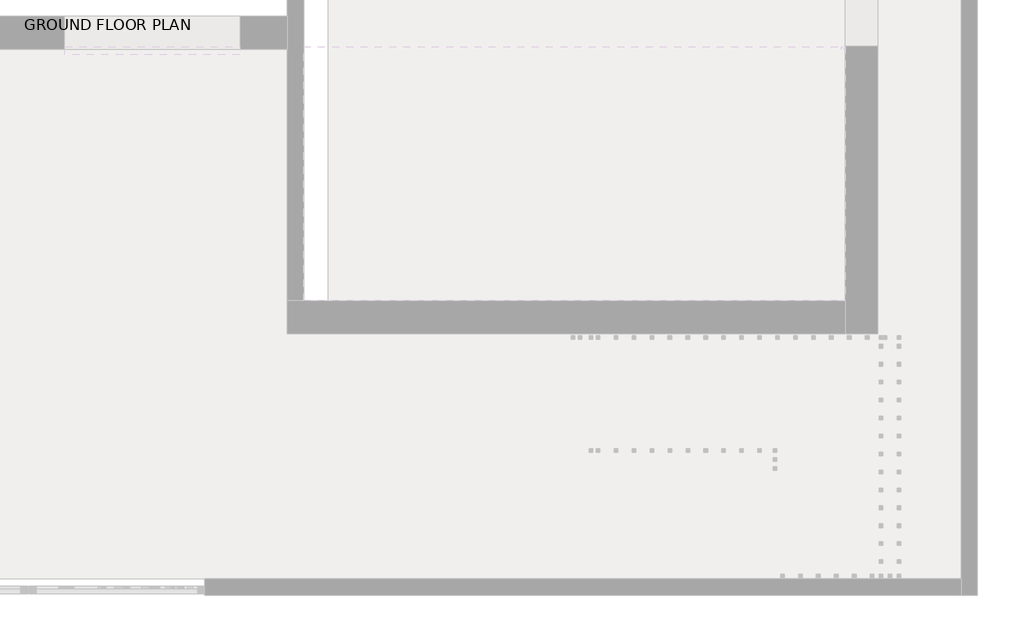
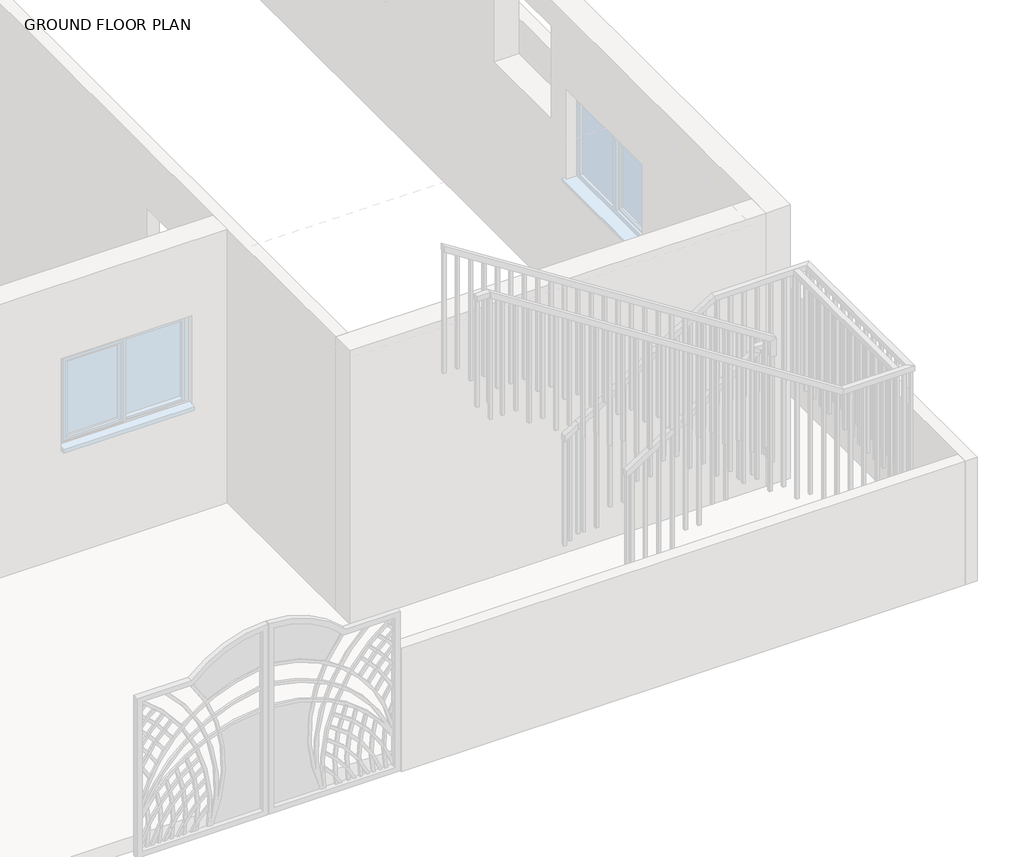
# One storey, part 14 of 23: 2 railings.
"""IFC4 building model written with IfcOpenShell, lengths in millimetres."""

from ifc_helpers import new_model, si_unit, frame, origin, place, context, project, spatial, polyline, outline, extrude, faceted_brep, element, save

model = new_model("IFC4")

# Units and contexts
model_context = context("Model", 3, world=origin())
ifc_project = project(units=[si_unit("LENGTHUNIT", "METRE", prefix="MILLI")], contexts=[model_context])

# Site, building, storey
site = spatial("IfcSite", under=ifc_project)
building = spatial("IfcBuilding", under=site)
storey = spatial("IfcBuildingStorey", under=building, Name="GROUND FLOOR PLAN", Elevation=487.68)

# Railings
placement = place(None, origin())
element("IfcRailing", 1, ObjectType="1100mm", at=placement, inside=storey, context=model_context, shape_type="SolidModel", body=[
    faceted_brep([(-8680.149573, -11007.9255223, 1912.8), (-8680.149573, -11007.9255223, 1853.4423995), (-8680.149573, -11057.9255223, 1853.4423995), (-8680.149573, -11057.9255223, 1912.8), (-7484.3306254, -11007.9255223, 2677.8717446), (-7434.3306254, -11007.9255223, 2650.5035914), (-7434.3306254, -11057.9255223, 2650.5035914), (-7484.3306254, -11057.9255223, 2677.8717446), (-7484.3306254, -11007.9255223, 2725.6), (-7434.3306254, -11007.9255223, 2675.6), (-7434.3306254, -11057.9255223, 2675.6), (-7484.3306254, -11057.9255223, 2725.6), (-7359.3306254, -11007.9255223, 2725.6), (-7359.3306254, -11007.9255223, 2675.6), (-7409.3306254, -11057.9255223, 2675.6), (-7409.3306254, -11057.9255223, 2725.6), (-7359.3306254, -11132.9255223, 2725.6), (-7359.3306254, -11132.9255223, 2675.6), (-7409.3306254, -11132.9255223, 2675.6), (-7409.3306254, -11132.9255223, 2725.6), (-7359.3306254, -11134.9255223, 2725.6), (-7409.3306254, -11134.9255223, 2725.6), (-7409.3306254, -11184.9255223, 2675.6), (-7359.3306254, -11184.9255223, 2675.6)], [[[0, 1, 2, 3]], [[1, 0, 4, 5]], [[2, 1, 5, 6]], [[3, 2, 6, 7]], [[0, 3, 7, 4]], [[5, 4, 8, 9]], [[6, 5, 9, 10]], [[7, 6, 10, 11]], [[4, 7, 11, 8]], [[9, 8, 12, 13]], [[10, 9, 13, 14]], [[11, 10, 14, 15]], [[8, 11, 15, 12]], [[13, 12, 16, 17]], [[14, 13, 17, 18]], [[15, 14, 18, 19]], [[12, 15, 19, 16]], [[20, 21, 22, 23]], [[17, 16, 20, 23]], [[18, 17, 23, 22]], [[19, 18, 22, 21]], [[16, 19, 21, 20]]]),
    faceted_brep([(-7359.3306254, -11134.9255223, 2725.6), (-7359.3306254, -11184.9255223, 2675.6), (-7409.3306254, -11184.9255223, 2675.6), (-7409.3306254, -11134.9255223, 2725.6), (-7359.3306254, -11134.9255223, 2855.9055527), (-7409.3306254, -11134.9255223, 2828.5415543), (-7409.3306254, -11184.9255223, 2828.5415543), (-7359.3306254, -11184.9255223, 2855.9055527)], [[[0, 1, 2, 3]], [[4, 5, 6, 7]], [[1, 0, 4, 7]], [[2, 1, 7, 6]], [[3, 2, 6, 5]], [[0, 3, 5, 4]]]),
    faceted_brep([(-7359.3306254, -11184.9255223, 2855.9055527), (-7409.3306254, -11184.9255223, 2828.5415543), (-7409.3306254, -11134.9255223, 2828.5415543), (-7359.3306254, -11134.9255223, 2855.9055527), (-10457.8773536, -11184.9255223, 4838.88), (-10457.8773536, -11134.9255223, 4838.88), (-10457.8773536, -11134.9255223, 4779.517542), (-10457.8773536, -11184.9255223, 4779.517542)], [[[0, 1, 2, 3]], [[4, 5, 6, 7]], [[1, 0, 4, 7]], [[2, 1, 7, 6]], [[3, 2, 6, 5]], [[0, 3, 5, 4]]]),
    extrude(outline(polyline([(3576.32, -10434.3306254), (4764.4483614, -10434.3306254), (4780.4475912, -10459.3306254), (3576.32, -10459.3306254), (3576.32, -10434.3306254)])), frame((0.0, -11172.4255223, 0.0), z_axis=(0.0, 1.0, 0.0), x_axis=(0.0, 0.0, 1.0)), (0.0, 0.0, 1.0), 25.0),
    extrude(outline(polyline([(3576.32, -10309.3306254), (4684.4522123, -10309.3306254), (4700.4514422, -10334.3306254), (3576.32, -10334.3306254), (3576.32, -10309.3306254)])), frame((0.0, -11172.4255223, 0.0), z_axis=(0.0, 1.0, 0.0), x_axis=(0.0, 0.0, 1.0)), (0.0, 0.0, 1.0), 25.0),
    extrude(outline(polyline([(3413.76, -10184.3306254), (4604.4560633, -10184.3306254), (4620.4552931, -10209.3306254), (3413.76, -10209.3306254), (3413.76, -10184.3306254)])), frame((0.0, -11172.4255223, 0.0), z_axis=(0.0, 1.0, 0.0), x_axis=(0.0, 0.0, 1.0)), (0.0, 0.0, 1.0), 25.0),
    extrude(outline(polyline([(3413.76, -10059.3306254), (4524.4599142, -10059.3306254), (4540.459144, -10084.3306254), (3413.76, -10084.3306254), (3413.76, -10059.3306254)])), frame((0.0, -11172.4255223, 0.0), z_axis=(0.0, 1.0, 0.0), x_axis=(0.0, 0.0, 1.0)), (0.0, 0.0, 1.0), 25.0),
    extrude(outline(polyline([(3251.2, -9934.3306254), (4444.4637652, -9934.3306254), (4460.462995, -9959.3306254), (3251.2, -9959.3306254), (3251.2, -9934.3306254)])), frame((0.0, -11172.4255223, 0.0), z_axis=(0.0, 1.0, 0.0), x_axis=(0.0, 0.0, 1.0)), (0.0, 0.0, 1.0), 25.0),
    extrude(outline(polyline([(3251.2, -9809.3306254), (4364.4676161, -9809.3306254), (4380.4668459, -9834.3306254), (3251.2, -9834.3306254), (3251.2, -9809.3306254)])), frame((0.0, -11172.4255223, 0.0), z_axis=(0.0, 1.0, 0.0), x_axis=(0.0, 0.0, 1.0)), (0.0, 0.0, 1.0), 25.0),
    extrude(outline(polyline([(3251.2, -9684.3306254), (4284.4714671, -9684.3306254), (4300.4706969, -9709.3306254), (3251.2, -9709.3306254), (3251.2, -9684.3306254)])), frame((0.0, -11172.4255223, 0.0), z_axis=(0.0, 1.0, 0.0), x_axis=(0.0, 0.0, 1.0)), (0.0, 0.0, 1.0), 25.0),
    extrude(outline(polyline([(3088.64, -9559.3306254), (4204.475318, -9559.3306254), (4220.4745478, -9584.3306254), (3088.64, -9584.3306254), (3088.64, -9559.3306254)])), frame((0.0, -11172.4255223, 0.0), z_axis=(0.0, 1.0, 0.0), x_axis=(0.0, 0.0, 1.0)), (0.0, 0.0, 1.0), 25.0),
    extrude(outline(polyline([(3088.64, -9434.3306254), (4124.479169, -9434.3306254), (4140.4783988, -9459.3306254), (3088.64, -9459.3306254), (3088.64, -9434.3306254)])), frame((0.0, -11172.4255223, 0.0), z_axis=(0.0, 1.0, 0.0), x_axis=(0.0, 0.0, 1.0)), (0.0, 0.0, 1.0), 25.0),
    extrude(outline(polyline([(2926.08, -9309.3306254), (4044.4830199, -9309.3306254), (4060.4822497, -9334.3306254), (2926.08, -9334.3306254), (2926.08, -9309.3306254)])), frame((0.0, -11172.4255223, 0.0), z_axis=(0.0, 1.0, 0.0), x_axis=(0.0, 0.0, 1.0)), (0.0, 0.0, 1.0), 25.0),
    extrude(outline(polyline([(2926.08, -9184.3306254), (3964.4868709, -9184.3306254), (3980.4861007, -9209.3306254), (2926.08, -9209.3306254), (2926.08, -9184.3306254)])), frame((0.0, -11172.4255223, 0.0), z_axis=(0.0, 1.0, 0.0), x_axis=(0.0, 0.0, 1.0)), (0.0, 0.0, 1.0), 25.0),
    extrude(outline(polyline([(2763.52, -9059.3306254), (3884.4907218, -9059.3306254), (3900.4899516, -9084.3306254), (2763.52, -9084.3306254), (2763.52, -9059.3306254)])), frame((0.0, -11172.4255223, 0.0), z_axis=(0.0, 1.0, 0.0), x_axis=(0.0, 0.0, 1.0)), (0.0, 0.0, 1.0), 25.0),
    extrude(outline(polyline([(2763.52, -8934.3306254), (3804.4945728, -8934.3306254), (3820.4938026, -8959.3306254), (2763.52, -8959.3306254), (2763.52, -8934.3306254)])), frame((0.0, -11172.4255223, 0.0), z_axis=(0.0, 1.0, 0.0), x_axis=(0.0, 0.0, 1.0)), (0.0, 0.0, 1.0), 25.0),
    extrude(outline(polyline([(2600.96, -8809.3306254), (3724.4984237, -8809.3306254), (3740.4976535, -8834.3306254), (2600.96, -8834.3306254), (2600.96, -8809.3306254)])), frame((0.0, -11172.4255223, 0.0), z_axis=(0.0, 1.0, 0.0), x_axis=(0.0, 0.0, 1.0)), (0.0, 0.0, 1.0), 25.0),
    extrude(outline(polyline([(2600.96, -8684.3306254), (3644.5022747, -8684.3306254), (3660.5015045, -8709.3306254), (2600.96, -8709.3306254), (2600.96, -8684.3306254)])), frame((0.0, -11172.4255223, 0.0), z_axis=(0.0, 1.0, 0.0), x_axis=(0.0, 0.0, 1.0)), (0.0, 0.0, 1.0), 25.0),
    extrude(outline(polyline([(2438.4, -8559.3306254), (3564.5061256, -8559.3306254), (3580.5053554, -8584.3306254), (2438.4, -8584.3306254), (2438.4, -8559.3306254)])), frame((0.0, -11172.4255223, 0.0), z_axis=(0.0, 1.0, 0.0), x_axis=(0.0, 0.0, 1.0)), (0.0, 0.0, 1.0), 25.0),
    extrude(outline(polyline([(2438.4, -8434.3306254), (3484.5099766, -8434.3306254), (3500.5092064, -8459.3306254), (2438.4, -8459.3306254), (2438.4, -8434.3306254)])), frame((0.0, -11172.4255223, 0.0), z_axis=(0.0, 1.0, 0.0), x_axis=(0.0, 0.0, 1.0)), (0.0, 0.0, 1.0), 25.0),
    extrude(outline(polyline([(2275.84, -8309.3306254), (3404.5138275, -8309.3306254), (3420.5130573, -8334.3306254), (2275.84, -8334.3306254), (2275.84, -8309.3306254)])), frame((0.0, -11172.4255223, 0.0), z_axis=(0.0, 1.0, 0.0), x_axis=(0.0, 0.0, 1.0)), (0.0, 0.0, 1.0), 25.0),
    extrude(outline(polyline([(2275.84, -8184.3306254), (3324.5176785, -8184.3306254), (3340.5169083, -8209.3306254), (2275.84, -8209.3306254), (2275.84, -8184.3306254)])), frame((0.0, -11172.4255223, 0.0), z_axis=(0.0, 1.0, 0.0), x_axis=(0.0, 0.0, 1.0)), (0.0, 0.0, 1.0), 25.0),
    extrude(outline(polyline([(2113.28, -8059.3306254), (3244.5215294, -8059.3306254), (3260.5207592, -8084.3306254), (2113.28, -8084.3306254), (2113.28, -8059.3306254)])), frame((0.0, -11172.4255223, 0.0), z_axis=(0.0, 1.0, 0.0), x_axis=(0.0, 0.0, 1.0)), (0.0, 0.0, 1.0), 25.0),
    extrude(outline(polyline([(2113.28, -7934.3306254), (3164.5253804, -7934.3306254), (3180.5246102, -7959.3306254), (2113.28, -7959.3306254), (2113.28, -7934.3306254)])), frame((0.0, -11172.4255223, 0.0), z_axis=(0.0, 1.0, 0.0), x_axis=(0.0, 0.0, 1.0)), (0.0, 0.0, 1.0), 25.0),
    extrude(outline(polyline([(1950.72, -7809.3306254), (3084.5292313, -7809.3306254), (3100.5284611, -7834.3306254), (1950.72, -7834.3306254), (1950.72, -7809.3306254)])), frame((0.0, -11172.4255223, 0.0), z_axis=(0.0, 1.0, 0.0), x_axis=(0.0, 0.0, 1.0)), (0.0, 0.0, 1.0), 25.0),
    extrude(outline(polyline([(1950.72, -7684.3306254), (3004.5330823, -7684.3306254), (3020.5323121, -7709.3306254), (1950.72, -7709.3306254), (1950.72, -7684.3306254)])), frame((0.0, -11172.4255223, 0.0), z_axis=(0.0, 1.0, 0.0), x_axis=(0.0, 0.0, 1.0)), (0.0, 0.0, 1.0), 25.0),
    extrude(outline(polyline([(1788.16, -7559.3306254), (2924.5369332, -7559.3306254), (2940.536163, -7584.3306254), (1788.16, -7584.3306254), (1788.16, -7559.3306254)])), frame((0.0, -11172.4255223, 0.0), z_axis=(0.0, 1.0, 0.0), x_axis=(0.0, 0.0, 1.0)), (0.0, 0.0, 1.0), 25.0),
    extrude(outline(polyline([(1788.16, -7434.3306254), (2844.5407841, -7434.3306254), (2860.540014, -7459.3306254), (1788.16, -7459.3306254), (1788.16, -7434.3306254)])), frame((0.0, -11172.4255223, 0.0), z_axis=(0.0, 1.0, 0.0), x_axis=(0.0, 0.0, 1.0)), (0.0, 0.0, 1.0), 25.0),
    extrude(outline(polyline([(-7396.8306254, -11082.9255223), (-7371.8306254, -11082.9255223), (-7371.8306254, -11107.9255223), (-7396.8306254, -11107.9255223), (-7396.8306254, -11082.9255223)])), frame((0.0, 0.0, 1625.6), z_axis=(0.0, 0.0, 1.0), x_axis=(1.0, 0.0, 0.0)), (0.0, 0.0, 1.0), 1050.0),
    extrude(outline(polyline([(2605.1944115, -7505.149573), (1463.04, -7505.149573), (1463.04, -7480.149573), (2621.1891352, -7480.149573), (2605.1944115, -7505.149573)])), frame((0.0, -11045.4255223, 0.0), z_axis=(0.0, 1.0, 0.0), x_axis=(0.0, 0.0, 1.0)), (0.0, 0.0, 1.0), 25.0),
    extrude(outline(polyline([(2525.2207932, -7630.149573), (1463.04, -7630.149573), (1463.04, -7605.149573), (2541.2155169, -7605.149573), (2525.2207932, -7630.149573)])), frame((0.0, -11045.4255223, 0.0), z_axis=(0.0, 1.0, 0.0), x_axis=(0.0, 0.0, 1.0)), (0.0, 0.0, 1.0), 25.0),
    extrude(outline(polyline([(2445.2471749, -7755.149573), (1300.48, -7755.149573), (1300.48, -7730.149573), (2461.2418986, -7730.149573), (2445.2471749, -7755.149573)])), frame((0.0, -11045.4255223, 0.0), z_axis=(0.0, 1.0, 0.0), x_axis=(0.0, 0.0, 1.0)), (0.0, 0.0, 1.0), 25.0),
    extrude(outline(polyline([(2365.2735566, -7880.149573), (1300.48, -7880.149573), (1300.48, -7855.149573), (2381.2682803, -7855.149573), (2365.2735566, -7880.149573)])), frame((0.0, -11045.4255223, 0.0), z_axis=(0.0, 1.0, 0.0), x_axis=(0.0, 0.0, 1.0)), (0.0, 0.0, 1.0), 25.0),
    extrude(outline(polyline([(2285.2999383, -8005.149573), (1137.92, -8005.149573), (1137.92, -7980.149573), (2301.294662, -7980.149573), (2285.2999383, -8005.149573)])), frame((0.0, -11045.4255223, 0.0), z_axis=(0.0, 1.0, 0.0), x_axis=(0.0, 0.0, 1.0)), (0.0, 0.0, 1.0), 25.0),
    extrude(outline(polyline([(2205.32632, -8130.149573), (1137.92, -8130.149573), (1137.92, -8105.149573), (2221.3210437, -8105.149573), (2205.32632, -8130.149573)])), frame((0.0, -11045.4255223, 0.0), z_axis=(0.0, 1.0, 0.0), x_axis=(0.0, 0.0, 1.0)), (0.0, 0.0, 1.0), 25.0),
    extrude(outline(polyline([(2125.3527017, -8255.149573), (975.36, -8255.149573), (975.36, -8230.149573), (2141.3474254, -8230.149573), (2125.3527017, -8255.149573)])), frame((0.0, -11045.4255223, 0.0), z_axis=(0.0, 1.0, 0.0), x_axis=(0.0, 0.0, 1.0)), (0.0, 0.0, 1.0), 25.0),
    extrude(outline(polyline([(2045.3790834, -8380.149573), (975.36, -8380.149573), (975.36, -8355.149573), (2061.3738071, -8355.149573), (2045.3790834, -8380.149573)])), frame((0.0, -11045.4255223, 0.0), z_axis=(0.0, 1.0, 0.0), x_axis=(0.0, 0.0, 1.0)), (0.0, 0.0, 1.0), 25.0),
    extrude(outline(polyline([(1965.4054651, -8505.149573), (812.8, -8505.149573), (812.8, -8480.149573), (1981.4001888, -8480.149573), (1965.4054651, -8505.149573)])), frame((0.0, -11045.4255223, 0.0), z_axis=(0.0, 1.0, 0.0), x_axis=(0.0, 0.0, 1.0)), (0.0, 0.0, 1.0), 25.0),
    extrude(outline(polyline([(1885.4318468, -8630.149573), (812.8, -8630.149573), (812.8, -8605.149573), (1901.4265705, -8605.149573), (1885.4318468, -8630.149573)])), frame((0.0, -11045.4255223, 0.0), z_axis=(0.0, 1.0, 0.0), x_axis=(0.0, 0.0, 1.0)), (0.0, 0.0, 1.0), 25.0),
    extrude(outline(polyline([(-7396.8306254, -11147.4255223), (-7371.8306254, -11147.4255223), (-7371.8306254, -11172.4255223), (-7396.8306254, -11172.4255223), (-7396.8306254, -11147.4255223)])), frame((0.0, 0.0, 1625.6), z_axis=(0.0, 0.0, 1.0), x_axis=(1.0, 0.0, 0.0)), (0.0, 0.0, 1.0), 1050.0),
    extrude(outline(polyline([(-7396.8306254, -11045.4255223), (-7396.8306254, -11020.4255223), (-7371.8306254, -11020.4255223), (-7371.8306254, -11045.4255223), (-7396.8306254, -11045.4255223)])), frame((0.0, 0.0, 1625.6), z_axis=(0.0, 0.0, 1.0), x_axis=(1.0, 0.0, 0.0)), (0.0, 0.0, 1.0), 1050.0),
    extrude(outline(polyline([(3576.32, -10432.8773536), (4763.5183122, -10432.8773536), (4779.517542, -10457.8773536), (3576.32, -10457.8773536), (3576.32, -10432.8773536)])), frame((0.0, -11172.4255223, 0.0), z_axis=(0.0, 1.0, 0.0), x_axis=(0.0, 0.0, 1.0)), (0.0, 0.0, 1.0), 25.0),
    extrude(outline(polyline([(1853.4423995, -8680.149573), (812.8, -8680.149573), (812.8, -8655.149573), (1869.4371231, -8655.149573), (1853.4423995, -8680.149573)])), frame((0.0, -11045.4255223, 0.0), z_axis=(0.0, 1.0, 0.0), x_axis=(0.0, 0.0, 1.0)), (0.0, 0.0, 1.0), 25.0),
])
element("IfcRailing", 2, ObjectType="1100mm", at=placement, inside=storey, context=model_context, shape_type="SolidModel", body=[
    faceted_brep([(-8680.149573, -10220.0521308, 1912.8), (-8680.149573, -10220.0521308, 1853.4423995), (-8680.149573, -10270.0521308, 1853.4423995), (-8680.149573, -10270.0521308, 1912.8), (-7409.7306254, -10220.0521308, 2725.6), (-7395.1045513, -10220.0521308, 2675.6), (-7395.1045513, -10270.0521308, 2675.6), (-7409.7306254, -10270.0521308, 2725.6), (-6495.8132565, -10220.0521308, 2725.6), (-6495.8132565, -10220.0521308, 2675.6), (-6545.8132565, -10270.0521308, 2675.6), (-6545.8132565, -10270.0521308, 2725.6), (-6495.8132565, -11933.6860066, 2725.6), (-6495.8132565, -11933.6860066, 2675.6), (-6545.8132565, -11883.6860066, 2675.6), (-6545.8132565, -11883.6860066, 2725.6), (-7155.718398, -11933.6860066, 2725.6), (-7170.3479429, -11933.6860066, 2675.6), (-7170.3479429, -11883.6860066, 2675.6), (-7155.718398, -11883.6860066, 2725.6), (-10457.8773536, -11933.6860066, 4838.88), (-10457.8773536, -11883.6860066, 4838.88), (-10457.8773536, -11883.6860066, 4779.517542), (-10457.8773536, -11933.6860066, 4779.517542)], [[[0, 1, 2, 3]], [[1, 0, 4, 5]], [[2, 1, 5, 6]], [[3, 2, 6, 7]], [[0, 3, 7, 4]], [[5, 4, 8, 9]], [[6, 5, 9, 10]], [[7, 6, 10, 11]], [[4, 7, 11, 8]], [[9, 8, 12, 13]], [[10, 9, 13, 14]], [[11, 10, 14, 15]], [[8, 11, 15, 12]], [[13, 12, 16, 17]], [[14, 13, 17, 18]], [[15, 14, 18, 19]], [[12, 15, 19, 16]], [[20, 21, 22, 23]], [[17, 16, 20, 23]], [[18, 17, 23, 22]], [[19, 18, 22, 21]], [[16, 19, 21, 20]]]),
    extrude(outline(polyline([(4691.8007425, -10320.8132565), (4707.7999723, -10345.8132565), (3576.32, -10345.8132565), (3576.32, -10320.8132565), (4691.8007425, -10320.8132565)])), frame((0.0, -11921.1860066, 0.0), z_axis=(0.0, 1.0, 0.0), x_axis=(0.0, 0.0, 1.0)), (0.0, 0.0, 1.0), 25.0),
    extrude(outline(polyline([(4611.8045935, -10195.8132565), (4627.8038233, -10220.8132565), (3576.32, -10220.8132565), (3576.32, -10195.8132565), (4611.8045935, -10195.8132565)])), frame((0.0, -11921.1860066, 0.0), z_axis=(0.0, 1.0, 0.0), x_axis=(0.0, 0.0, 1.0)), (0.0, 0.0, 1.0), 25.0),
    extrude(outline(polyline([(4531.8084444, -10070.8132565), (4547.8076742, -10095.8132565), (3413.76, -10095.8132565), (3413.76, -10070.8132565), (4531.8084444, -10070.8132565)])), frame((0.0, -11921.1860066, 0.0), z_axis=(0.0, 1.0, 0.0), x_axis=(0.0, 0.0, 1.0)), (0.0, 0.0, 1.0), 25.0),
    extrude(outline(polyline([(4451.8122954, -9945.8132565), (4467.8115252, -9970.8132565), (3413.76, -9970.8132565), (3413.76, -9945.8132565), (4451.8122954, -9945.8132565)])), frame((0.0, -11921.1860066, 0.0), z_axis=(0.0, 1.0, 0.0), x_axis=(0.0, 0.0, 1.0)), (0.0, 0.0, 1.0), 25.0),
    extrude(outline(polyline([(4371.8161463, -9820.8132565), (4387.8153761, -9845.8132565), (3251.2, -9845.8132565), (3251.2, -9820.8132565), (4371.8161463, -9820.8132565)])), frame((0.0, -11921.1860066, 0.0), z_axis=(0.0, 1.0, 0.0), x_axis=(0.0, 0.0, 1.0)), (0.0, 0.0, 1.0), 25.0),
    extrude(outline(polyline([(4291.8423995, -9695.8132565), (4307.8371231, -9720.8132565), (3251.2, -9720.8132565), (3251.2, -9695.8132565), (4291.8423995, -9695.8132565)])), frame((0.0, -11921.1860066, 0.0), z_axis=(0.0, 1.0, 0.0), x_axis=(0.0, 0.0, 1.0)), (0.0, 0.0, 1.0), 25.0),
    extrude(outline(polyline([(4211.8238482, -9570.8132565), (4227.823078, -9595.8132565), (3088.64, -9595.8132565), (3088.64, -9570.8132565), (4211.8238482, -9570.8132565)])), frame((0.0, -11921.1860066, 0.0), z_axis=(0.0, 1.0, 0.0), x_axis=(0.0, 0.0, 1.0)), (0.0, 0.0, 1.0), 25.0),
    extrude(outline(polyline([(4131.8276992, -9445.8132565), (4147.826929, -9470.8132565), (3088.64, -9470.8132565), (3088.64, -9445.8132565), (4131.8276992, -9445.8132565)])), frame((0.0, -11921.1860066, 0.0), z_axis=(0.0, 1.0, 0.0), x_axis=(0.0, 0.0, 1.0)), (0.0, 0.0, 1.0), 25.0),
    extrude(outline(polyline([(4051.8315501, -9320.8132565), (4067.8307799, -9345.8132565), (2926.08, -9345.8132565), (2926.08, -9320.8132565), (4051.8315501, -9320.8132565)])), frame((0.0, -11921.1860066, 0.0), z_axis=(0.0, 1.0, 0.0), x_axis=(0.0, 0.0, 1.0)), (0.0, 0.0, 1.0), 25.0),
    extrude(outline(polyline([(3971.835401, -9195.8132565), (3987.8346309, -9220.8132565), (2926.08, -9220.8132565), (2926.08, -9195.8132565), (3971.835401, -9195.8132565)])), frame((0.0, -11921.1860066, 0.0), z_axis=(0.0, 1.0, 0.0), x_axis=(0.0, 0.0, 1.0)), (0.0, 0.0, 1.0), 25.0),
    extrude(outline(polyline([(3891.839252, -9070.8132565), (3907.8384818, -9095.8132565), (2763.52, -9095.8132565), (2763.52, -9070.8132565), (3891.839252, -9070.8132565)])), frame((0.0, -11921.1860066, 0.0), z_axis=(0.0, 1.0, 0.0), x_axis=(0.0, 0.0, 1.0)), (0.0, 0.0, 1.0), 25.0),
    extrude(outline(polyline([(3811.8431029, -8945.8132565), (3827.8423328, -8970.8132565), (2763.52, -8970.8132565), (2763.52, -8945.8132565), (3811.8431029, -8945.8132565)])), frame((0.0, -11921.1860066, 0.0), z_axis=(0.0, 1.0, 0.0), x_axis=(0.0, 0.0, 1.0)), (0.0, 0.0, 1.0), 25.0),
    extrude(outline(polyline([(3731.8469539, -8820.8132565), (3747.8461837, -8845.8132565), (2600.96, -8845.8132565), (2600.96, -8820.8132565), (3731.8469539, -8820.8132565)])), frame((0.0, -11921.1860066, 0.0), z_axis=(0.0, 1.0, 0.0), x_axis=(0.0, 0.0, 1.0)), (0.0, 0.0, 1.0), 25.0),
    extrude(outline(polyline([(3651.8508048, -8695.8132565), (3667.8500347, -8720.8132565), (2600.96, -8720.8132565), (2600.96, -8695.8132565), (3651.8508048, -8695.8132565)])), frame((0.0, -11921.1860066, 0.0), z_axis=(0.0, 1.0, 0.0), x_axis=(0.0, 0.0, 1.0)), (0.0, 0.0, 1.0), 25.0),
    extrude(outline(polyline([(3571.8546558, -8570.8132565), (3587.8538856, -8595.8132565), (2438.4, -8595.8132565), (2438.4, -8570.8132565), (3571.8546558, -8570.8132565)])), frame((0.0, -11921.1860066, 0.0), z_axis=(0.0, 1.0, 0.0), x_axis=(0.0, 0.0, 1.0)), (0.0, 0.0, 1.0), 25.0),
    extrude(outline(polyline([(3491.8585067, -8445.8132565), (3507.8577365, -8470.8132565), (2438.4, -8470.8132565), (2438.4, -8445.8132565), (3491.8585067, -8445.8132565)])), frame((0.0, -11921.1860066, 0.0), z_axis=(0.0, 1.0, 0.0), x_axis=(0.0, 0.0, 1.0)), (0.0, 0.0, 1.0), 25.0),
    extrude(outline(polyline([(3411.8623577, -8320.8132565), (3427.8615875, -8345.8132565), (2275.84, -8345.8132565), (2275.84, -8320.8132565), (3411.8623577, -8320.8132565)])), frame((0.0, -11921.1860066, 0.0), z_axis=(0.0, 1.0, 0.0), x_axis=(0.0, 0.0, 1.0)), (0.0, 0.0, 1.0), 25.0),
    extrude(outline(polyline([(3331.8662086, -8195.8132565), (3347.8654384, -8220.8132565), (2275.84, -8220.8132565), (2275.84, -8195.8132565), (3331.8662086, -8195.8132565)])), frame((0.0, -11921.1860066, 0.0), z_axis=(0.0, 1.0, 0.0), x_axis=(0.0, 0.0, 1.0)), (0.0, 0.0, 1.0), 25.0),
    extrude(outline(polyline([(3251.8700596, -8070.8132565), (3267.8692894, -8095.8132565), (2113.28, -8095.8132565), (2113.28, -8070.8132565), (3251.8700596, -8070.8132565)])), frame((0.0, -11921.1860066, 0.0), z_axis=(0.0, 1.0, 0.0), x_axis=(0.0, 0.0, 1.0)), (0.0, 0.0, 1.0), 25.0),
    extrude(outline(polyline([(3171.8739105, -7945.8132565), (3187.8731403, -7970.8132565), (2113.28, -7970.8132565), (2113.28, -7945.8132565), (3171.8739105, -7945.8132565)])), frame((0.0, -11921.1860066, 0.0), z_axis=(0.0, 1.0, 0.0), x_axis=(0.0, 0.0, 1.0)), (0.0, 0.0, 1.0), 25.0),
    extrude(outline(polyline([(3091.8777615, -7820.8132565), (3107.8769913, -7845.8132565), (1950.72, -7845.8132565), (1950.72, -7820.8132565), (3091.8777615, -7820.8132565)])), frame((0.0, -11921.1860066, 0.0), z_axis=(0.0, 1.0, 0.0), x_axis=(0.0, 0.0, 1.0)), (0.0, 0.0, 1.0), 25.0),
    extrude(outline(polyline([(3011.8816124, -7695.8132565), (3027.8808422, -7720.8132565), (1950.72, -7720.8132565), (1950.72, -7695.8132565), (3011.8816124, -7695.8132565)])), frame((0.0, -11921.1860066, 0.0), z_axis=(0.0, 1.0, 0.0), x_axis=(0.0, 0.0, 1.0)), (0.0, 0.0, 1.0), 25.0),
    extrude(outline(polyline([(2931.8854634, -7570.8132565), (2947.8846932, -7595.8132565), (1788.16, -7595.8132565), (1788.16, -7570.8132565), (2931.8854634, -7570.8132565)])), frame((0.0, -11921.1860066, 0.0), z_axis=(0.0, 1.0, 0.0), x_axis=(0.0, 0.0, 1.0)), (0.0, 0.0, 1.0), 25.0),
    extrude(outline(polyline([(2851.8893143, -7445.8132565), (2867.8885441, -7470.8132565), (1788.16, -7470.8132565), (1788.16, -7445.8132565), (2851.8893143, -7445.8132565)])), frame((0.0, -11921.1860066, 0.0), z_axis=(0.0, 1.0, 0.0), x_axis=(0.0, 0.0, 1.0)), (0.0, 0.0, 1.0), 25.0),
    extrude(outline(polyline([(2771.8931653, -7320.8132565), (2787.8923951, -7345.8132565), (1625.6, -7345.8132565), (1625.6, -7320.8132565), (2771.8931653, -7320.8132565)])), frame((0.0, -11921.1860066, 0.0), z_axis=(0.0, 1.0, 0.0), x_axis=(0.0, 0.0, 1.0)), (0.0, 0.0, 1.0), 25.0),
    extrude(outline(polyline([(2691.8970162, -7195.8132565), (2707.896246, -7220.8132565), (1625.6, -7220.8132565), (1625.6, -7195.8132565), (2691.8970162, -7195.8132565)])), frame((0.0, -11921.1860066, 0.0), z_axis=(0.0, 1.0, 0.0), x_axis=(0.0, 0.0, 1.0)), (0.0, 0.0, 1.0), 25.0),
    extrude(outline(polyline([(-7070.8132565, -11921.1860066), (-7095.8132565, -11921.1860066), (-7095.8132565, -11896.1860066), (-7070.8132565, -11896.1860066), (-7070.8132565, -11921.1860066)])), frame((0.0, 0.0, 1625.6), z_axis=(0.0, 0.0, 1.0), x_axis=(1.0, 0.0, 0.0)), (0.0, 0.0, 1.0), 1050.0),
    extrude(outline(polyline([(-6945.8132565, -11921.1860066), (-6970.8132565, -11921.1860066), (-6970.8132565, -11896.1860066), (-6945.8132565, -11896.1860066), (-6945.8132565, -11921.1860066)])), frame((0.0, 0.0, 1625.6), z_axis=(0.0, 0.0, 1.0), x_axis=(1.0, 0.0, 0.0)), (0.0, 0.0, 1.0), 1050.0),
    extrude(outline(polyline([(-6820.8132565, -11921.1860066), (-6845.8132565, -11921.1860066), (-6845.8132565, -11896.1860066), (-6820.8132565, -11896.1860066), (-6820.8132565, -11921.1860066)])), frame((0.0, 0.0, 1625.6), z_axis=(0.0, 0.0, 1.0), x_axis=(1.0, 0.0, 0.0)), (0.0, 0.0, 1.0), 1050.0),
    extrude(outline(polyline([(-6695.8132565, -11921.1860066), (-6720.8132565, -11921.1860066), (-6720.8132565, -11896.1860066), (-6695.8132565, -11896.1860066), (-6695.8132565, -11921.1860066)])), frame((0.0, 0.0, 1625.6), z_axis=(0.0, 0.0, 1.0), x_axis=(1.0, 0.0, 0.0)), (0.0, 0.0, 1.0), 1050.0),
    extrude(outline(polyline([(-6570.8132565, -11921.1860066), (-6595.8132565, -11921.1860066), (-6595.8132565, -11896.1860066), (-6570.8132565, -11896.1860066), (-6570.8132565, -11921.1860066)])), frame((0.0, 0.0, 1625.6), z_axis=(0.0, 0.0, 1.0), x_axis=(1.0, 0.0, 0.0)), (0.0, 0.0, 1.0), 1050.0),
    extrude(outline(polyline([(-6508.3132565, -11795.0521308), (-6508.3132565, -11820.0521308), (-6533.3132565, -11820.0521308), (-6533.3132565, -11795.0521308), (-6508.3132565, -11795.0521308)])), frame((0.0, 0.0, 1625.6), z_axis=(0.0, 0.0, 1.0), x_axis=(1.0, 0.0, 0.0)), (0.0, 0.0, 1.0), 1050.0),
    extrude(outline(polyline([(-6508.3132565, -11670.0521308), (-6508.3132565, -11695.0521308), (-6533.3132565, -11695.0521308), (-6533.3132565, -11670.0521308), (-6508.3132565, -11670.0521308)])), frame((0.0, 0.0, 1625.6), z_axis=(0.0, 0.0, 1.0), x_axis=(1.0, 0.0, 0.0)), (0.0, 0.0, 1.0), 1050.0),
    extrude(outline(polyline([(-6508.3132565, -11545.0521308), (-6508.3132565, -11570.0521308), (-6533.3132565, -11570.0521308), (-6533.3132565, -11545.0521308), (-6508.3132565, -11545.0521308)])), frame((0.0, 0.0, 1625.6), z_axis=(0.0, 0.0, 1.0), x_axis=(1.0, 0.0, 0.0)), (0.0, 0.0, 1.0), 1050.0),
    extrude(outline(polyline([(-6508.3132565, -11420.0521308), (-6508.3132565, -11445.0521308), (-6533.3132565, -11445.0521308), (-6533.3132565, -11420.0521308), (-6508.3132565, -11420.0521308)])), frame((0.0, 0.0, 1625.6), z_axis=(0.0, 0.0, 1.0), x_axis=(1.0, 0.0, 0.0)), (0.0, 0.0, 1.0), 1050.0),
    extrude(outline(polyline([(-6508.3132565, -11295.0521308), (-6508.3132565, -11320.0521308), (-6533.3132565, -11320.0521308), (-6533.3132565, -11295.0521308), (-6508.3132565, -11295.0521308)])), frame((0.0, 0.0, 1625.6), z_axis=(0.0, 0.0, 1.0), x_axis=(1.0, 0.0, 0.0)), (0.0, 0.0, 1.0), 1050.0),
    extrude(outline(polyline([(-6508.3132565, -11170.0521308), (-6508.3132565, -11195.0521308), (-6533.3132565, -11195.0521308), (-6533.3132565, -11170.0521308), (-6508.3132565, -11170.0521308)])), frame((0.0, 0.0, 1625.6), z_axis=(0.0, 0.0, 1.0), x_axis=(1.0, 0.0, 0.0)), (0.0, 0.0, 1.0), 1050.0),
    extrude(outline(polyline([(-6508.3132565, -11045.0521308), (-6508.3132565, -11070.0521308), (-6533.3132565, -11070.0521308), (-6533.3132565, -11045.0521308), (-6508.3132565, -11045.0521308)])), frame((0.0, 0.0, 1625.6), z_axis=(0.0, 0.0, 1.0), x_axis=(1.0, 0.0, 0.0)), (0.0, 0.0, 1.0), 1050.0),
    extrude(outline(polyline([(-6508.3132565, -10920.0521308), (-6508.3132565, -10945.0521308), (-6533.3132565, -10945.0521308), (-6533.3132565, -10920.0521308), (-6508.3132565, -10920.0521308)])), frame((0.0, 0.0, 1625.6), z_axis=(0.0, 0.0, 1.0), x_axis=(1.0, 0.0, 0.0)), (0.0, 0.0, 1.0), 1050.0),
    extrude(outline(polyline([(-6508.3132565, -10795.0521308), (-6508.3132565, -10820.0521308), (-6533.3132565, -10820.0521308), (-6533.3132565, -10795.0521308), (-6508.3132565, -10795.0521308)])), frame((0.0, 0.0, 1625.6), z_axis=(0.0, 0.0, 1.0), x_axis=(1.0, 0.0, 0.0)), (0.0, 0.0, 1.0), 1050.0),
    extrude(outline(polyline([(-6508.3132565, -10670.0521308), (-6508.3132565, -10695.0521308), (-6533.3132565, -10695.0521308), (-6533.3132565, -10670.0521308), (-6508.3132565, -10670.0521308)])), frame((0.0, 0.0, 1625.6), z_axis=(0.0, 0.0, 1.0), x_axis=(1.0, 0.0, 0.0)), (0.0, 0.0, 1.0), 1050.0),
    extrude(outline(polyline([(-6508.3132565, -10545.0521308), (-6508.3132565, -10570.0521308), (-6533.3132565, -10570.0521308), (-6533.3132565, -10545.0521308), (-6508.3132565, -10545.0521308)])), frame((0.0, 0.0, 1625.6), z_axis=(0.0, 0.0, 1.0), x_axis=(1.0, 0.0, 0.0)), (0.0, 0.0, 1.0), 1050.0),
    extrude(outline(polyline([(-6508.3132565, -10420.0521308), (-6508.3132565, -10445.0521308), (-6533.3132565, -10445.0521308), (-6533.3132565, -10420.0521308), (-6508.3132565, -10420.0521308)])), frame((0.0, 0.0, 1625.6), z_axis=(0.0, 0.0, 1.0), x_axis=(1.0, 0.0, 0.0)), (0.0, 0.0, 1.0), 1050.0),
    extrude(outline(polyline([(-6508.3132565, -10295.0521308), (-6508.3132565, -10320.0521308), (-6533.3132565, -10320.0521308), (-6533.3132565, -10295.0521308), (-6508.3132565, -10295.0521308)])), frame((0.0, 0.0, 1625.6), z_axis=(0.0, 0.0, 1.0), x_axis=(1.0, 0.0, 0.0)), (0.0, 0.0, 1.0), 1050.0),
    extrude(outline(polyline([(-6630.149573, -10232.5521308), (-6605.149573, -10232.5521308), (-6605.149573, -10257.5521308), (-6630.149573, -10257.5521308), (-6630.149573, -10232.5521308)])), frame((0.0, 0.0, 1625.6), z_axis=(0.0, 0.0, 1.0), x_axis=(1.0, 0.0, 0.0)), (0.0, 0.0, 1.0), 1050.0),
    extrude(outline(polyline([(-6755.149573, -10232.5521308), (-6730.149573, -10232.5521308), (-6730.149573, -10257.5521308), (-6755.149573, -10257.5521308), (-6755.149573, -10232.5521308)])), frame((0.0, 0.0, 1625.6), z_axis=(0.0, 0.0, 1.0), x_axis=(1.0, 0.0, 0.0)), (0.0, 0.0, 1.0), 1050.0),
    extrude(outline(polyline([(-6880.149573, -10232.5521308), (-6855.149573, -10232.5521308), (-6855.149573, -10257.5521308), (-6880.149573, -10257.5521308), (-6880.149573, -10232.5521308)])), frame((0.0, 0.0, 1625.6), z_axis=(0.0, 0.0, 1.0), x_axis=(1.0, 0.0, 0.0)), (0.0, 0.0, 1.0), 1050.0),
    extrude(outline(polyline([(-7005.149573, -10232.5521308), (-6980.149573, -10232.5521308), (-6980.149573, -10257.5521308), (-7005.149573, -10257.5521308), (-7005.149573, -10232.5521308)])), frame((0.0, 0.0, 1625.6), z_axis=(0.0, 0.0, 1.0), x_axis=(1.0, 0.0, 0.0)), (0.0, 0.0, 1.0), 1050.0),
    extrude(outline(polyline([(-7130.149573, -10232.5521308), (-7105.149573, -10232.5521308), (-7105.149573, -10257.5521308), (-7130.149573, -10257.5521308), (-7130.149573, -10232.5521308)])), frame((0.0, 0.0, 1625.6), z_axis=(0.0, 0.0, 1.0), x_axis=(1.0, 0.0, 0.0)), (0.0, 0.0, 1.0), 1050.0),
    extrude(outline(polyline([(-7255.149573, -10232.5521308), (-7230.149573, -10232.5521308), (-7230.149573, -10257.5521308), (-7255.149573, -10257.5521308), (-7255.149573, -10232.5521308)])), frame((0.0, 0.0, 1625.6), z_axis=(0.0, 0.0, 1.0), x_axis=(1.0, 0.0, 0.0)), (0.0, 0.0, 1.0), 1050.0),
    extrude(outline(polyline([(-7380.149573, -10232.5521308), (-7355.149573, -10232.5521308), (-7355.149573, -10257.5521308), (-7380.149573, -10257.5521308), (-7380.149573, -10232.5521308)])), frame((0.0, 0.0, 1625.6), z_axis=(0.0, 0.0, 1.0), x_axis=(1.0, 0.0, 0.0)), (0.0, 0.0, 1.0), 1050.0),
    extrude(outline(polyline([(1463.04, -7505.149573), (1463.04, -7480.149573), (2621.1891352, -7480.149573), (2605.1944115, -7505.149573), (1463.04, -7505.149573)])), frame((0.0, -10257.5521308, 0.0), z_axis=(0.0, 1.0, 0.0), x_axis=(0.0, 0.0, 1.0)), (0.0, 0.0, 1.0), 25.0),
    extrude(outline(polyline([(1463.04, -7630.149573), (1463.04, -7605.149573), (2541.2155169, -7605.149573), (2525.2207932, -7630.149573), (1463.04, -7630.149573)])), frame((0.0, -10257.5521308, 0.0), z_axis=(0.0, 1.0, 0.0), x_axis=(0.0, 0.0, 1.0)), (0.0, 0.0, 1.0), 25.0),
    extrude(outline(polyline([(1300.48, -7755.149573), (1300.48, -7730.149573), (2461.2418986, -7730.149573), (2445.2471749, -7755.149573), (1300.48, -7755.149573)])), frame((0.0, -10257.5521308, 0.0), z_axis=(0.0, 1.0, 0.0), x_axis=(0.0, 0.0, 1.0)), (0.0, 0.0, 1.0), 25.0),
    extrude(outline(polyline([(1300.48, -7880.149573), (1300.48, -7855.149573), (2381.2682803, -7855.149573), (2365.2735566, -7880.149573), (1300.48, -7880.149573)])), frame((0.0, -10257.5521308, 0.0), z_axis=(0.0, 1.0, 0.0), x_axis=(0.0, 0.0, 1.0)), (0.0, 0.0, 1.0), 25.0),
    extrude(outline(polyline([(1137.92, -8005.149573), (1137.92, -7980.149573), (2301.294662, -7980.149573), (2285.2999383, -8005.149573), (1137.92, -8005.149573)])), frame((0.0, -10257.5521308, 0.0), z_axis=(0.0, 1.0, 0.0), x_axis=(0.0, 0.0, 1.0)), (0.0, 0.0, 1.0), 25.0),
    extrude(outline(polyline([(1137.92, -8130.149573), (1137.92, -8105.149573), (2221.3210437, -8105.149573), (2205.32632, -8130.149573), (1137.92, -8130.149573)])), frame((0.0, -10257.5521308, 0.0), z_axis=(0.0, 1.0, 0.0), x_axis=(0.0, 0.0, 1.0)), (0.0, 0.0, 1.0), 25.0),
    extrude(outline(polyline([(975.36, -8255.149573), (975.36, -8230.149573), (2141.3474254, -8230.149573), (2125.3527017, -8255.149573), (975.36, -8255.149573)])), frame((0.0, -10257.5521308, 0.0), z_axis=(0.0, 1.0, 0.0), x_axis=(0.0, 0.0, 1.0)), (0.0, 0.0, 1.0), 25.0),
    extrude(outline(polyline([(975.36, -8380.149573), (975.36, -8355.149573), (2061.3738071, -8355.149573), (2045.3790834, -8380.149573), (975.36, -8380.149573)])), frame((0.0, -10257.5521308, 0.0), z_axis=(0.0, 1.0, 0.0), x_axis=(0.0, 0.0, 1.0)), (0.0, 0.0, 1.0), 25.0),
    extrude(outline(polyline([(812.8, -8505.149573), (812.8, -8480.149573), (1981.4001888, -8480.149573), (1965.4054651, -8505.149573), (812.8, -8505.149573)])), frame((0.0, -10257.5521308, 0.0), z_axis=(0.0, 1.0, 0.0), x_axis=(0.0, 0.0, 1.0)), (0.0, 0.0, 1.0), 25.0),
    extrude(outline(polyline([(812.8, -8630.149573), (812.8, -8605.149573), (1901.4265705, -8605.149573), (1885.4318468, -8630.149573), (812.8, -8630.149573)])), frame((0.0, -10257.5521308, 0.0), z_axis=(0.0, 1.0, 0.0), x_axis=(0.0, 0.0, 1.0)), (0.0, 0.0, 1.0), 25.0),
    extrude(outline(polyline([(-6508.3132565, -11896.1860066), (-6508.3132565, -11921.1860066), (-6533.3132565, -11921.1860066), (-6533.3132565, -11896.1860066), (-6508.3132565, -11896.1860066)])), frame((0.0, 0.0, 1625.6), z_axis=(0.0, 0.0, 1.0), x_axis=(1.0, 0.0, 0.0)), (0.0, 0.0, 1.0), 1050.0),
    extrude(outline(polyline([(-6533.3132565, -10232.5521308), (-6508.3132565, -10232.5521308), (-6508.3132565, -10257.5521308), (-6533.3132565, -10257.5521308), (-6533.3132565, -10232.5521308)])), frame((0.0, 0.0, 1625.6), z_axis=(0.0, 0.0, 1.0), x_axis=(1.0, 0.0, 0.0)), (0.0, 0.0, 1.0), 1050.0),
    extrude(outline(polyline([(4763.5183122, -10432.8773536), (4779.517542, -10457.8773536), (3576.32, -10457.8773536), (3576.32, -10432.8773536), (4763.5183122, -10432.8773536)])), frame((0.0, -11921.1860066, 0.0), z_axis=(0.0, 1.0, 0.0), x_axis=(0.0, 0.0, 1.0)), (0.0, 0.0, 1.0), 25.0),
    extrude(outline(polyline([(812.8, -8680.149573), (812.8, -8655.149573), (1869.4371231, -8655.149573), (1853.4423995, -8680.149573), (812.8, -8680.149573)])), frame((0.0, -10257.5521308, 0.0), z_axis=(0.0, 1.0, 0.0), x_axis=(0.0, 0.0, 1.0)), (0.0, 0.0, 1.0), 25.0),
])

save(model, "model.ifc")

# Revit data of these elements
# Type "1100mm"
#   built-in parameter 1008612 = 0.019685 (stored number, unit not read)
#   built-in parameter 1008611 = 0.019685 (stored number, unit not read)
#   built-in parameter 1008609 = 0.902231 (stored number, unit not read)
#   built-in parameter 1008604 = 0.19685 (stored number, unit not read)
#   built-in parameter 1008603 = 0.164042 (stored number, unit not read)
#   Railing Height = 3.608924 ft
#   built-in parameter 1008630 = 2
#   built-in parameter 1008610 = 2
#   built-in parameter 1008608 = 1
#   built-in parameter 1008618 = Baluster_Square : 25mm
# Elements 1, 2 (IfcRailing, "1100mm")
#   Phase Created = New Construction
